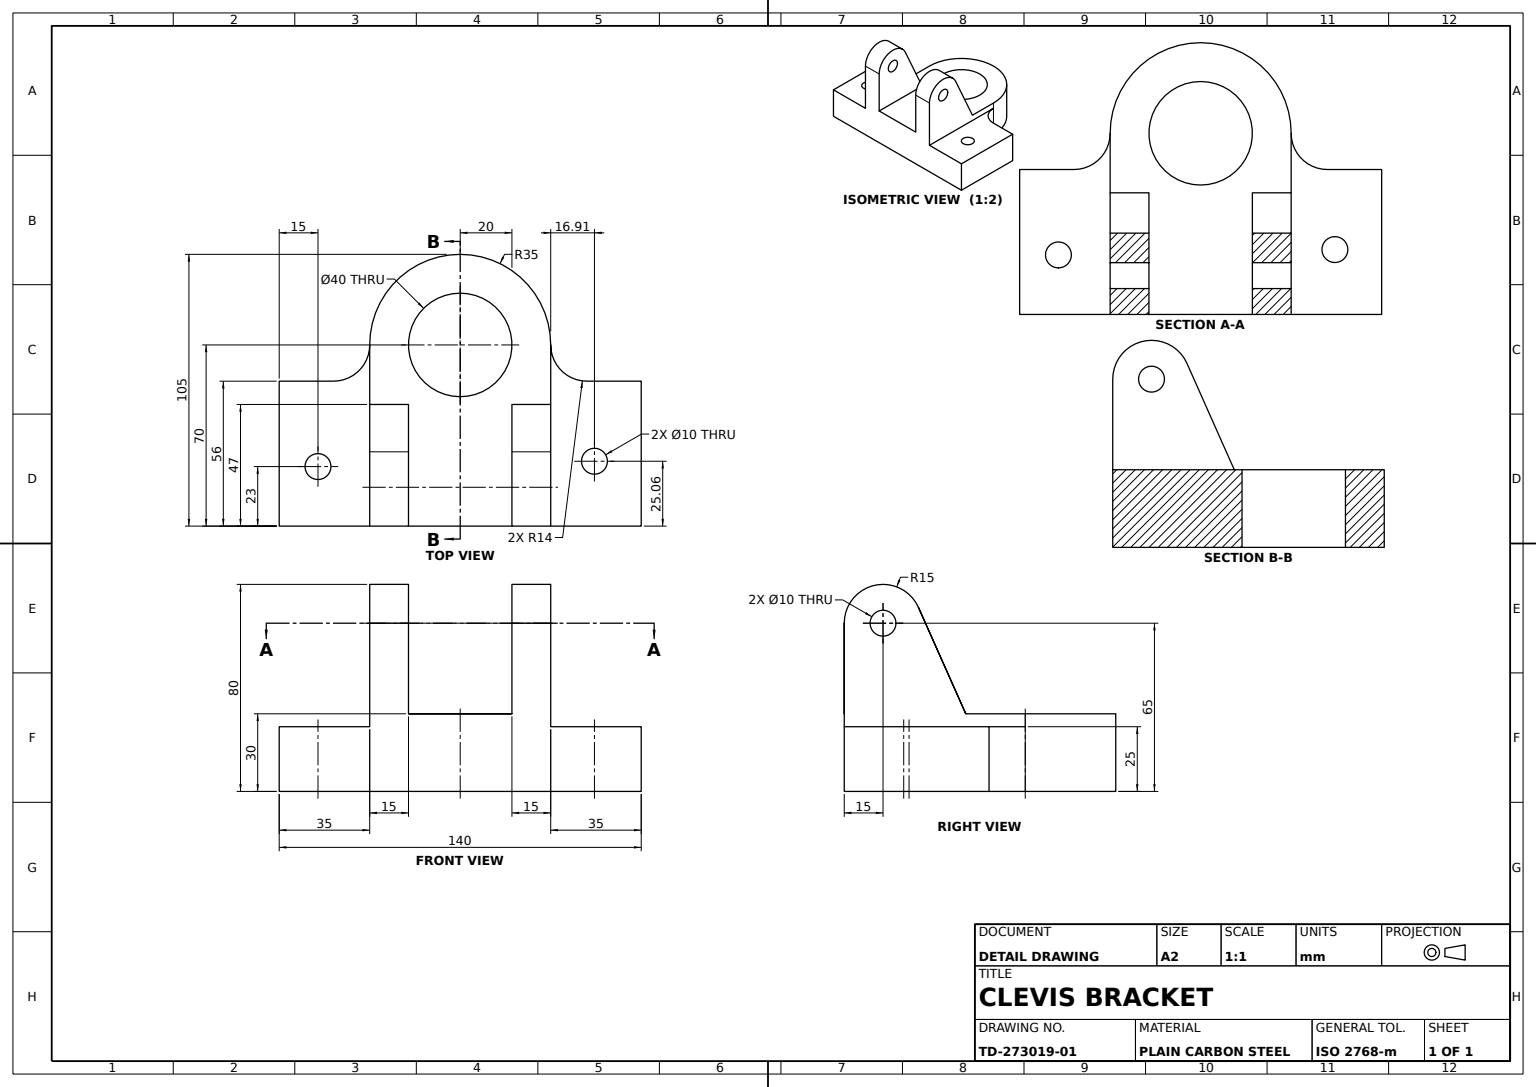
from build123d import *

# Parameters (mm, degrees)
BASE_PLATE_DEPTH               = 25
HOUSING_PROFILE_CUT_DEPTH      = 61
HOUSING_PROFILE_CUT_DEPTH_BACK = 91
HOUSING_BOSS_DEPTH             = 5
BORE_40_DEPTH                  = 110
BORE_40_DEPTH_BACK             = 116
BORE_40_SKETCH_R               = 20
MOUNTING_HOLE_10_A_SKETCH_R    = 5
MOUNTING_HOLE_10_A_DEPTH       = 393
MOUNTING_HOLE_10_B_DEPTH       = 393
MOUNTING_HOLE_10_B_DEPTH_BACK  = 393
MOUNTING_HOLE_10_B_SKETCH_R    = 5
CLEVIS_LUGS_DEPTH              = 70
LUG_GAP_CUT_SKETCH_W           = 40
LUG_GAP_CUT_SKETCH_H           = 47
LUG_GAP_CUT_DEPTH              = 207
PIN_HOLE_10_DEPTH              = 207
PIN_HOLE_10_DEPTH_BACK         = 207
PIN_HOLE_10_SKETCH_R           = 5


with BuildPart() as part:
    # Base Plate Sketch → Base Plate (new body)
    with BuildSketch(Plane(origin=(0, 0, 0), x_dir=(1, 0, 0), z_dir=(0, 1, 0))):
        Polygon((-70, 95.100325632), (70, 95.100325632), (70, 73.269753582), (70, -31.730246418), (-70, -31.730246418), (-70, 73.269753582), align=None)
    extrude(amount=BASE_PLATE_DEPTH)

    # Housing Profile Cut Sketch → Housing Profile Cut (cut, two sides: drawn at the far end of the back side and taken through both)
    with BuildSketch(Plane(origin=(0, 25, 0), x_dir=(1, 0, 0), z_dir=(0, 1, 0)).offset(-HOUSING_PROFILE_CUT_DEPTH_BACK)):
        with BuildLine():
            Line((49, 24.269753582), (70, 24.269753582))
            Line((70, 24.269753582), (70, 95.100325632))
            Line((70, 95.100325632), (-70, 95.100325632))
            Line((-70, 95.100325632), (-70, 24.269753582))
            Line((-70, 24.269753582), (-49, 24.269753582))
            ThreePointArc((-49, 24.269753582), (-39.100505063, 28.370258646), (-35, 38.269753582))
            ThreePointArc((-35, 38.269753582), (0, 73.269753582), (35, 38.269753582))
            ThreePointArc((35, 38.269753582), (39.100505063, 28.370258646), (49, 24.269753582))
        make_face()
    extrude(amount=HOUSING_PROFILE_CUT_DEPTH + HOUSING_PROFILE_CUT_DEPTH_BACK, mode=Mode.SUBTRACT)

    # Housing Boss Sketch → Housing Boss (add)
    with BuildSketch(Plane(origin=(0, 25, 0), x_dir=(1, 0, 0), z_dir=(0, 1, 0))):
        with BuildLine():
            ThreePointArc((-35, 38.269753582), (0, 3.269753582), (35, 38.269753582))
            ThreePointArc((35, 38.269753582), (0, 73.269753582), (-35, 38.269753582))
        make_face()
        with BuildLine():
            Line((35, -31.730246418), (35, 38.269753582))
            ThreePointArc((35, 38.269753582), (0, 3.269753582), (-35, 38.269753582))
            Line((-35, 38.269753582), (-35, -31.730246418))
            Line((-35, -31.730246418), (35, -31.730246418))
        make_face()
    extrude(amount=HOUSING_BOSS_DEPTH)

    # Bore Ø40 Sketch → Bore Ø40 (cut, two sides: drawn at the far end of the back side and taken through both)
    with BuildSketch(Plane(origin=(0, 30, 0), x_dir=(1, 0, 0), z_dir=(0, 1, 0)).offset(-BORE_40_DEPTH_BACK)):
        with Locations(Location((0, 38.269753582, 0), (0, 0, 90))):
            Circle(BORE_40_SKETCH_R)
    extrude(amount=BORE_40_DEPTH + BORE_40_DEPTH_BACK, mode=Mode.SUBTRACT)

    # Mounting Hole Ø10 A Sketch → Mounting Hole Ø10 A (cut)
    with BuildSketch(Plane(origin=(0, 25, 0), x_dir=(1, 0, 0), z_dir=(0, 1, 0))):
        with Locations(Location((-55, -8.730246418, 0), (0, 0, 270))):
            Circle(MOUNTING_HOLE_10_A_SKETCH_R)
    extrude(amount=-MOUNTING_HOLE_10_A_DEPTH, mode=Mode.SUBTRACT)

    # Mounting Hole Ø10 B Sketch → Mounting Hole Ø10 B (cut, two sides: drawn at the far end of the back side and taken through both)
    with BuildSketch(Plane(origin=(0, 25, 0), x_dir=(1, 0, 0), z_dir=(0, 1, 0)).offset(-MOUNTING_HOLE_10_B_DEPTH_BACK)):
        with Locations(Location((51.913967656, -6.666465324, 0), (0, 0, 90))):
            Circle(MOUNTING_HOLE_10_B_SKETCH_R)
    extrude(amount=MOUNTING_HOLE_10_B_DEPTH + MOUNTING_HOLE_10_B_DEPTH_BACK, mode=Mode.SUBTRACT)

    # Clevis Lugs Sketch → Clevis Lugs (add)
    with BuildSketch(Plane(origin=(35, 0, 0), x_dir=(0, 0, -1), z_dir=(1, 0, 0))):
        with BuildLine():
            Line((-31.730246418, 65), (-31.730246418, 30))
            Line((-31.730246418, 30), (15.269753582, 30))
            Line((15.269753582, 30), (-3.026748887, 71.100340599))
            ThreePointArc((-3.026748887, 71.100340599), (-19.84854219, 79.67229469), (-31.730246418, 65))
        make_face()
    extrude(amount=-CLEVIS_LUGS_DEPTH)

    # Lug Gap Cut Sketch → Lug Gap Cut (cut)
    with BuildSketch(Plane(origin=(0, 30, 0), x_dir=(1, 0, 0), z_dir=(0, 1, 0))):
        with Locations((0, -8.230246418)):
            Rectangle(LUG_GAP_CUT_SKETCH_W, LUG_GAP_CUT_SKETCH_H)
    extrude(amount=LUG_GAP_CUT_DEPTH, mode=Mode.SUBTRACT)

    # Pin Hole Ø10 Sketch → Pin Hole Ø10 (cut, two sides: drawn at the far end of the back side and taken through both)
    with BuildSketch(Plane.ZY.offset(35).offset(-PIN_HOLE_10_DEPTH_BACK)):
        with Locations(Location((16.730246418, 65, 0), (0, 0, 180))):
            Circle(PIN_HOLE_10_SKETCH_R)
    extrude(amount=PIN_HOLE_10_DEPTH + PIN_HOLE_10_DEPTH_BACK, mode=Mode.SUBTRACT)


solid = part.part
